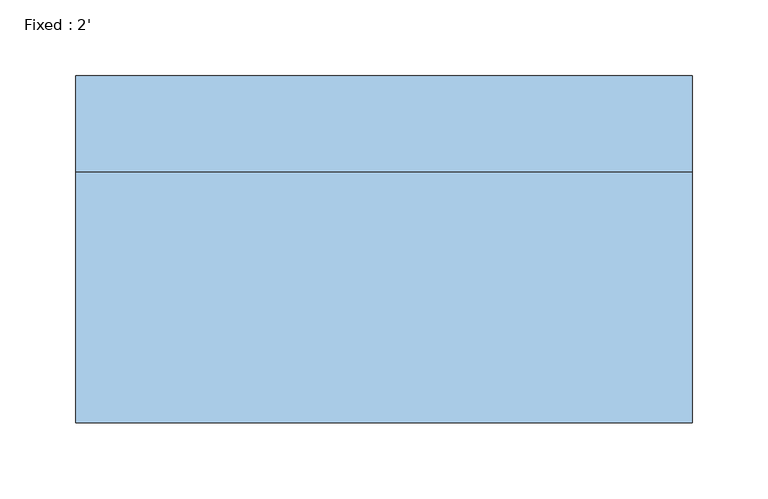
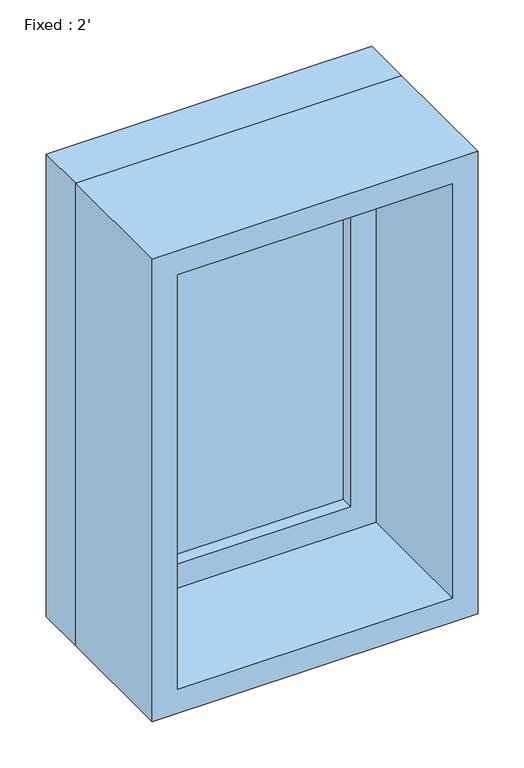
"""IFC4 building model written with IfcOpenShell, lengths in millimetres: window geometry, Fixed : 2'."""

from ifc_helpers import new_model, si_unit, frame, origin, place, context, project, spatial, polyline, outline, extrude, source, transform, mapped, element, save


def fixed_2_415b3208(model_context):
    return source(origin(), model_context, "Body", "SweptSolid", [
        extrude(outline(polyline([(101.6, 66.675), (-177.8, 66.675), (-177.8, 79.375), (101.6, 79.375), (101.6, 66.675)])), frame((0.0, 0.0, 368.3), z_axis=(0.0, 0.0, 1.0), x_axis=(1.0, 0.0, 0.0)), (0.0, 0.0, 1.0), 482.6),
        extrude(outline(polyline([(895.35, -222.25), (323.85, -222.25), (323.85, 146.05), (895.35, 146.05), (895.35, -222.25)]), holes=[polyline([(850.9, -177.8), (850.9, 101.6), (368.3, 101.6), (368.3, -177.8), (850.9, -177.8)])]), frame((0.0, 50.8, 0.0), z_axis=(0.0, 1.0, 0.0), x_axis=(0.0, 0.0, 1.0)), (0.0, 0.0, 1.0), 44.45),
        extrude(outline(polyline([(914.4, -241.3), (304.8, -241.3), (304.8, 165.1), (914.4, 165.1), (914.4, -241.3)]), holes=[polyline([(882.65, -209.55), (882.65, 133.35), (336.55, 133.35), (336.55, -209.55), (882.65, -209.55)])]), frame((0.0, -114.3, 0.0), z_axis=(0.0, 1.0, 0.0), x_axis=(0.0, 0.0, 1.0)), (0.0, 0.0, 1.0), 165.1),
        extrude(outline(polyline([(914.4, 165.1), (914.4, -241.3), (304.8, -241.3), (304.8, 165.1), (914.4, 165.1)]), holes=[polyline([(895.35, 146.05), (323.85, 146.05), (323.85, -222.25), (895.35, -222.25), (895.35, 146.05)])]), frame((0.0, 50.8, 0.0), z_axis=(0.0, 1.0, 0.0), x_axis=(0.0, 0.0, 1.0)), (0.0, 0.0, 1.0), 63.5),
    ])


if __name__ == "__main__":
    model = new_model("IFC4")
    model_context = context("Model", 3, world=origin())
    ifc_project = project(units=[si_unit("LENGTHUNIT", "METRE", prefix="MILLI")], contexts=[model_context])
    site = spatial("IfcSite", under=ifc_project)
    building = spatial("IfcBuilding", under=site)
    placement = place(None, origin())
    fixed_2_shape = fixed_2_415b3208(model_context)
    element("IfcWindow", 1, ObjectType="Fixed : 2'", at=placement, inside=building, context=model_context, shape_type="MappedRepresentation", body=[
        mapped(fixed_2_shape, transform((0.0, 0.0, 0.0), x_axis=(1.0, 0.0, 0.0), y_axis=(0.0, 1.0, 0.0), z_axis=(0.0, 0.0, 1.0))),
    ])
    save(model, "model.ifc")

# Revit data of these elements
# Type "Fixed : 2'"
#   Type Mark = "20"
#   Construction Type Id = "GSP4R"
#   Assembly Code = "B2020100"
#   Analytic Construction = "1/8 in Pilkington single glazing"
#   Visual Light Transmittance = 0.9
#   Solar Heat Gain Coefficient = 0.78
#   Heat Transfer Coefficient (U) = 0.6496 BTU/(h·ft²·°F)
#   Height = 2' - 0"
#   Default Sill Height = 1' - 0"
#   Width = 1' - 4"
#   Window Inset = 0' - 0 3/4"
#   Define Thermal Properties by = 1
#   Glass Pane Material = Glass
#   Sash Material = Sash
#   Wall Closure = (empty or 0)
# Element 1 (IfcWindow, "Fixed : 2'")
#   Materials on its faces: "Sash", "Glass"
# Materials
#   "Glass": class "Glass", colour RGB 0 128 192, transparency 0.75, Description = "Soda Lime Glass", Cost = 0
#   "Sash": class "Wood", colour RGB 224 178 126, transparency 0, Cost = 0
